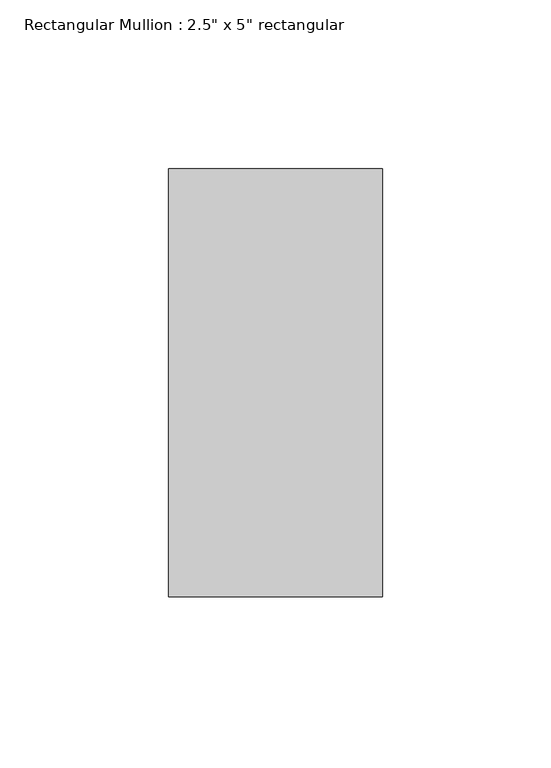
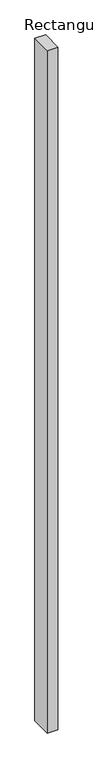
"""IFC4 building model written with IfcOpenShell, lengths in millimetres: member geometry."""

from ifc_helpers import new_model, si_unit, frame, origin, place, context, project, spatial, polyline, outline, extrude, source, transform, mapped, element, save


def member_4da692ab(model_context):
    return source(origin(), model_context, "Body", "SweptSolid", [
        extrude(outline(polyline([(0.0, 63.5), (0.0, -63.5), (-63.5, -63.5), (-63.5, 63.5), (0.0, 63.5)])), frame((0.0, 0.0, -4292.6), z_axis=(0.0, 0.0, 1.0), x_axis=(1.0, 0.0, 0.0)), (0.0, 0.0, 1.0), 4292.6),
    ])


if __name__ == "__main__":
    model = new_model("IFC4")
    model_context = context("Model", 3, world=origin())
    ifc_project = project(units=[si_unit("LENGTHUNIT", "METRE", prefix="MILLI")], contexts=[model_context])
    site = spatial("IfcSite", under=ifc_project)
    building = spatial("IfcBuilding", under=site)
    placement = place(None, origin())
    member_shape = member_4da692ab(model_context)
    element("IfcMember", 1, ObjectType="Rectangular Mullion : 2.5\" x 5\" rectangular", at=placement, inside=building, context=model_context, shape_type="MappedRepresentation", body=[
        mapped(member_shape, transform((0.0, 0.0, 0.0), x_axis=(1.0, 0.0, 0.0), y_axis=(0.0, 1.0, 0.0), z_axis=(0.0, 0.0, 1.0))),
    ])
    save(model, "model.ifc")

# Revit data of these elements
# Type "Rectangular Mullion : 2.5\" x 5\" rectangular"
#   built-in parameter 1007304 = 0.416667 (stored number, unit not read)
#   built-in parameter 1007301 = 0.104167 (stored number, unit not read)
#   built-in parameter 1007300 = 0.104167 (stored number, unit not read)
# Element 1 (IfcMember, "Rectangular Mullion : 2.5\" x 5\" rectangular")
#   Materials on its faces: "Aluminum"
# Materials
#   "Aluminum": class "Metal", colour RGB 247 247 247, transparency 0, Description = "Aluminum 6061", Cost = 0
